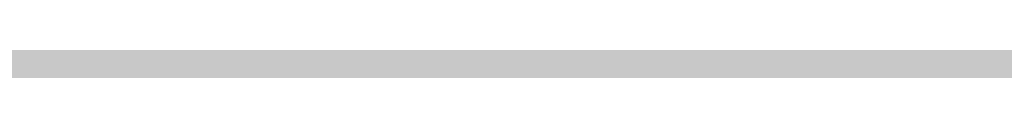
# Model space of a CAD drawing. Units: feet. Extents: x 3168 to 4724, y 827 to 1477.
# Tile 86 of 256: x 3274.148 to 3275.224, y 1099.001 to 1099.015. Entities that reach past the tile are written whole.
import ezdxf

# ---------------------------------------------------------------- set-up
doc = ezdxf.new("R2010")
doc.units = ezdxf.units.FT
doc.layers.add('A-ELEV', color=7, linetype='Continuous', lineweight=35)
doc.layers.add('A-ELEV-PATT', color=8, linetype='Continuous', lineweight=13)

msp = doc.modelspace()

# ---------------------------------------------------------------- hatches: boundary and pattern name
at = {"layer": 'A-ELEV-PATT'}
h = msp.add_hatch(color=256, dxfattribs=at)
h.dxf.hatch_style = 1
edge = h.paths.add_edge_path()
edge.add_ellipse((3552.9058, 979.2201), major_axis=(36.7449, 0), ratio=0.4848485, start_angle=0, end_angle=360)
edge = h.paths.add_edge_path()
edge.add_ellipse((3559.8916, 929.2523), major_axis=(36.7449, 0), ratio=0.4848485, start_angle=0, end_angle=360)
edge = h.paths.add_edge_path()
edge.add_line((3299.3168, 1198.6061), (3479.9167, 1198.6061))
edge.add_line((3479.9167, 1198.6061), (3479.9167, 1209.8686))
edge.add_spline(control_points=[(3479.9167, 1209.8686), (3464.3012, 1209.8686), (3448.6856, 1209.8686), (3410.9491, 1209.8686), (3388.8282, 1209.8686), (3355.6469, 1209.8686), (3344.5864, 1209.8686), (3327.9957, 1209.8686), (3322.4655, 1209.8686), (3314.1702, 1209.8686), (3311.4051, 1209.8686), (3307.2574, 1209.8686), (3305.8748, 1209.8686), (3303.801, 1209.8686), (3303.1097, 1209.8686), (3302.0728, 1209.8686), (3301.7272, 1209.8686), (3301.2087, 1209.8686), (3301.0359, 1209.8686), (3300.7767, 1209.8686), (3300.6903, 1209.8686), (3300.5606, 1209.8686), (3300.5174, 1209.8686), (3300.4526, 1209.8686), (3300.431, 1209.8686), (3300.3986, 1209.8686), (3300.3878, 1209.8686), (3300.3662, 1209.8686), (3300.3457, 1209.8686), (3300.3455, 1209.8686), (3300.3455, 1209.8686), (3300.3433, 1209.8686), (3300.3411, 1209.8686), (3300.3379, 1209.8686), (3300.3368, 1209.8686), (3300.3339, 1209.8686), (3300.3321, 1209.8686), (3300.3255, 1209.8686), (3300.3207, 1209.8686), (3300.3109, 1209.8686), (3300.306, 1209.8686), (3300.2905, 1209.8686), (3300.28, 1209.8686), (3300.2324, 1209.8688), (3300.1953, 1209.869), (3299.9511, 1209.8706), (3299.7448, 1209.8743), (3299.4368, 1209.8833), (3299.3344, 1209.8868), (3299.1811, 1209.8929), (3299.13, 1209.8951), (3298.6522, 1209.9168), (3298.2295, 1209.9457), (3297.6016, 1210.0024), (3297.3934, 1210.0235), (3297.0827, 1210.0583), (3296.9793, 1210.0705), (3296.293, 1210.1549), (3295.7181, 1210.2434), (3294.8687, 1210.3989), (3294.5877, 1210.4545), (3294.1693, 1210.5433), (3294.0304, 1210.5739), (3291.7071, 1211.1012), (3289.6536, 1211.8134), (3285.7763, 1213.564), (3283.9514, 1214.6035), (3280.5122, 1216.9801), (3278.8972, 1218.3176), (3276.3799, 1220.8295), (3275.416, 1221.9177), (3274.0393, 1223.7077), (3273.581, 1224.3495), (3273.1432, 1225.0163)], knot_values=[39.119033, 39.119033, 39.119033, 39.119033, 39.286353, 39.286353, 39.523379, 39.523379, 39.641892, 39.641892, 39.701148, 39.701148, 39.730777, 39.730777, 39.745591, 39.745591, 39.752998, 39.752998, 39.756701, 39.756701, 39.758553, 39.758553, 39.759479, 39.759479, 39.759942, 39.759942, 39.760173, 39.760173, 39.760289, 39.760289, 39.760405, 39.760405, 39.760463, 39.760463, 39.763389, 39.763389, 39.764851, 39.764851, 39.767304, 39.767304, 39.773825, 39.773825, 39.78057, 39.78057, 39.79477, 39.79477, 39.845194, 39.845194, 40.126715, 40.126715, 40.267476, 40.267476, 40.337856, 40.337856, 40.927023, 40.927023, 41.221606, 41.221606, 41.368898, 41.368898, 42.202622, 42.202622, 42.619485, 42.619485, 42.827916, 42.827916, 46.118323, 46.118323, 49.408731, 49.408731, 52.699139, 52.699139, 54.927489, 54.927489, 56.104228, 56.104228, 56.104228, 56.104228], weights=[1, 1, 1, 1, 1, 1, 1, 1, 1, 1, 1, 1, 1, 1, 1, 1, 1, 1, 1, 1, 1, 1, 1, 1, 1, 1, 1, 1, 1, 1, 1, 1, 1, 1, 1, 1, 1, 1, 1, 1, 1, 1, 1, 1, 1, 1, 1, 1, 1, 1, 1, 1, 1, 1, 1, 1, 1, 1, 1, 1, 1, 1, 1, 1, 1, 1, 1, 1, 1, 1, 1, 1, 1, 1], degree=3, periodic=0)
edge.add_line((3273.1432, 1225.0163), (3273.1432, 1099.0163))
edge.add_line((3273.1432, 1099.0163), (3299.3168, 1099.0163))
edge.add_line((3299.3168, 1099.0163), (3299.3168, 1198.6061))
edge = h.paths.add_edge_path()
edge.add_line((3304.7584, 1324.1581), (3479.9167, 1324.1581))
edge.add_line((3479.9167, 1324.1581), (3479.9167, 1335.7146))
edge.add_line((3479.9167, 1335.7146), (3269.1616, 1335.7146))
edge.add_spline(control_points=[(3269.1616, 1335.7146), (3264.0242, 1335.7146), (3258.3641, 1328.9582), (3259.2643, 1323.9003)], knot_values=[0, 0, 0, 0, 15.412191, 15.412191, 15.412191, 15.412191], degree=3, periodic=0)
edge.add_line((3259.2643, 1323.9003), (3265.5168, 1288.7691))
edge.add_line((3265.5168, 1288.7691), (3275.2651, 1261.5456))
edge.add_line((3275.2651, 1261.5456), (3304.7584, 1261.5456))
edge.add_line((3304.7584, 1261.5456), (3304.7584, 1324.1581))
h = msp.add_hatch(color=256, dxfattribs=at)
h.dxf.hatch_style = 1
h.paths.add_polyline_path([(3384.5252, 1099.0163), (3335.0292, 1099.0163), (3299.3168, 1099.0163), (3273.1432, 1099.0163), (3217.5654, 1099.0163), (3168.0693, 827.1163), (3335.0292, 827.1163)])

# ---------------------------------------------------------------- linework, layer by layer
at = {"layer": 'A-ELEV'}
msp.add_open_spline([(3808.5202, 1099.0163), (3808.5202, 1141.4132), (3808.5202, 1183.8102), (3808.5202, 1226.6353), (3808.5202, 1227.0636), (3808.5202, 1227.4918), (3811.4919, 1248.9947), (3814.4635, 1270.4975), (3817.4652, 1292.2176), (3817.4952, 1292.4348), (3817.5253, 1292.652), (3817.5728, 1310.1067), (3817.6203, 1327.5615), (3817.6679, 1345.0163), (3817.6679, 1345.458), (3817.6679, 1345.8996), (3817.6679, 1346.456), (3817.6679, 1346.5708), (3817.6679, 1346.7529), (3817.6679, 1346.8201), (3817.6679, 1346.9349), (3817.6679, 1346.9823), (3817.6679, 1347.0386), (3817.6679, 1347.0474), (3817.6679, 1347.0737), (3817.6679, 1347.0593), (3817.6679, 1347.0615), (3817.6679, 1347.0627), (3817.6679, 1347.066), (3817.6679, 1347.0683), (3817.6679, 1347.075), (3817.6679, 1347.0795), (3817.6678, 1347.0929), (3817.6678, 1347.1019), (3817.6678, 1347.1288), (3817.6677, 1347.1467), (3817.6674, 1347.2004), (3817.6672, 1347.2362), (3817.6661, 1347.3434), (3817.665, 1347.4147), (3817.6608, 1347.6281), (3817.6566, 1347.7697), (3817.64, 1348.1925), (3817.6235, 1348.4716), (3817.5591, 1349.3001), (3817.4961, 1349.8406), (3817.2554, 1351.4242), (3817.0263, 1352.4288), (3816.3069, 1354.8889), (3815.7437, 1356.2687), (3814.464, 1358.8192), (3813.7464, 1359.991), (3812.1958, 1362.1723), (3811.3622, 1363.1821), (3809.5888, 1365.069), (3808.6488, 1365.9461), (3806.6543, 1367.5796), (3805.5997, 1368.3362), (3803.3529, 1369.7223), (3802.1605, 1370.3524), (3799.6008, 1371.4536), (3798.2327, 1371.9255), (3795.2801, 1372.6346), (3793.6931, 1372.8721), (3791.8694, 1372.9265), (3791.7409, 1372.9292), (3791.3534, 1372.9341), (3791.0927, 1372.9329), (3790.3041, 1372.9151), (3789.7695, 1372.8842), (3789.2092, 1372.8302), (3789.1906, 1372.8284), (3789.1349, 1372.8229), (3789.0977, 1372.8191), (3789.0484, 1372.814), (3789.0364, 1372.8127), (3789.0003, 1372.8089), (3788.9761, 1372.8063), (3788.9494, 1372.8034), (3788.9468, 1372.8031), (3788.9426, 1372.8027), (3788.941, 1372.8025), (3788.9386, 1372.8022), (3788.9378, 1372.8021), (3788.9354, 1372.8019), (3788.8675, 1372.7944), (3788.7569, 1372.7822), (3788.7015, 1372.7761), (3788.5355, 1372.7579), (3788.4249, 1372.7457), (3788.0929, 1372.7092), (3787.8715, 1372.6848), (3787.2075, 1372.6118), (3786.7648, 1372.5631), (3785.4368, 1372.417), (3784.5515, 1372.3196), (3781.8954, 1372.0274), (3780.1247, 1371.8327), (3774.8126, 1371.2483), (3771.2713, 1370.8587), (3760.6471, 1369.69), (3753.5643, 1368.9109), (3732.316, 1366.5735), (3718.1504, 1365.0152), (3694.0068, 1362.3593), (3684.0287, 1361.2617), (3674.0506, 1360.1641), (3664.6007, 1360.1641), (3655.1508, 1360.1641), (3626.8011, 1360.1641), (3607.9013, 1360.1641), (3551.2019, 1360.1641), (3513.4023, 1360.1641), (3467.7252, 1360.1641), (3459.8476, 1360.1641), (3436.2149, 1360.1641), (3420.4597, 1360.1641), (3373.1943, 1360.1641), (3341.6839, 1360.1641), (3302.8482, 1360.1641), (3295.5227, 1360.1641), (3286.0383, 1360.1641), (3283.8794, 1360.1641), (3277.4026, 1360.1641), (3273.0848, 1360.1641), (3267.7329, 1360.1641), (3266.6988, 1360.1641), (3263.5965, 1360.1641), (3261.5284, 1360.1641), (3259.2369, 1360.1641), (3259.0137, 1360.1641), (3258.344, 1360.1641), (3257.8975, 1360.1641), (3257.431, 1360.1641), (3257.411, 1360.1641), (3257.3706, 1360.1641), (3257.3755, 1360.1641), (3257.3746, 1360.1641), (3257.3739, 1360.1641), (3257.372, 1360.1641), (3257.3706, 1360.1641), (3257.3667, 1360.1641), (3257.364, 1360.1641), (3257.3561, 1360.1641), (3257.3508, 1360.164), (3257.335, 1360.164), (3257.3244, 1360.164), (3257.2928, 1360.1639), (3257.2717, 1360.1638), (3257.2084, 1360.1634), (3257.1663, 1360.163), (3257.0402, 1360.1614), (3256.9563, 1360.1598), (3256.7055, 1360.1534), (3256.5392, 1360.147), (3256.0436, 1360.1219), (3255.7173, 1360.0971), (3254.7524, 1360.0005), (3254.128, 1359.9065), (3252.1801, 1359.5253), (3250.9416, 1359.144), (3248.6702, 1358.2433), (3247.6357, 1357.7238), (3245.7326, 1356.6035), (3244.8634, 1356.0021), (3243.2531, 1354.7429), (3242.512, 1354.0847), (3240.7511, 1352.3448), (3239.801, 1351.2296), (3238.0878, 1348.8724), (3237.3247, 1347.6304), (3235.9825, 1344.9716), (3235.4022, 1343.5549), (3234.5911, 1340.8155), (3234.3109, 1339.5435), (3233.9765, 1336.8026), (3233.9221, 1335.3309), (3234.1489, 1332.5913), (3234.3495, 1331.3672), (3234.7199, 1329.9994), (3234.7524, 1329.8834), (3234.8536, 1329.5348), (3234.9259, 1329.3017), (3235.0248, 1329.0026), (3235.0469, 1328.9369), (3235.0776, 1328.8472), (3235.0859, 1328.8232), (3235.1109, 1328.7511), (3235.1278, 1328.703), (3235.148, 1328.6462), (3235.1511, 1328.6376), (3235.1561, 1328.6235), (3235.1581, 1328.618), (3235.1602, 1328.612), (3235.1656, 1328.5969), (3235.1801, 1328.5565), (3235.1903, 1328.5281), (3235.2208, 1328.4429), (3235.2411, 1328.3862), (3235.3021, 1328.2159), (3235.3427, 1328.1023), (3235.4647, 1327.7617), (3235.546, 1327.5346), (3235.79, 1326.8534), (3235.9526, 1326.3992), (3236.4405, 1325.0367), (3236.7657, 1324.1284), (3237.7415, 1321.4034), (3238.392, 1319.5868), (3240.3435, 1314.1369), (3241.6445, 1310.5036), (3245.5476, 1299.6037), (3248.1496, 1292.3371), (3255.9557, 1270.5374), (3261.1598, 1256.0042), (3267.3876, 1238.612), (3268.4114, 1235.7529), (3269.5104, 1232.6839), (3269.5856, 1232.4739), (3269.7066, 1232.1359), (3269.7524, 1232.0079), (3269.8273, 1231.7987), (3269.8564, 1231.7176), (3269.9063, 1231.5781), (3269.9272, 1231.5198), (3269.9725, 1231.3934), (3269.9968, 1231.3254), (3270.0265, 1231.2425), (3270.0318, 1231.2277), (3270.0403, 1231.204), (3270.0392, 1231.207), (3270.0394, 1231.2066), (3270.0394, 1231.2064), (3270.0396, 1231.2058), (3270.0398, 1231.2055), (3270.0402, 1231.2043), (3270.0404, 1231.2036), (3270.0413, 1231.2013), (3270.0418, 1231.1998), (3270.0434, 1231.1953), (3270.0445, 1231.1922), (3270.0478, 1231.1832), (3270.0499, 1231.1771), (3270.0564, 1231.159), (3270.0608, 1231.147), (3270.0739, 1231.1108), (3270.0826, 1231.0867), (3270.1089, 1231.0144), (3270.1266, 1230.9663), (3270.1799, 1230.8225), (3270.2159, 1230.7269), (3270.3253, 1230.4415), (3270.4, 1230.2528), (3270.6292, 1229.6914), (3270.7889, 1229.3235), (3271.2865, 1228.2383), (3271.6431, 1227.5398), (3272.7759, 1225.5153), (3273.6142, 1224.2605), (3275.416, 1221.9177), (3276.3799, 1220.8295), (3278.8972, 1218.3176), (3280.5122, 1216.9801), (3283.9514, 1214.6035), (3285.7763, 1213.564), (3289.6536, 1211.8134), (3291.7071, 1211.1012), (3294.0304, 1210.5739), (3294.1693, 1210.5433), (3294.5877, 1210.4545), (3294.8687, 1210.3989), (3295.7181, 1210.2434), (3296.293, 1210.1549), (3296.9793, 1210.0705), (3297.0827, 1210.0583), (3297.3934, 1210.0235), (3297.6016, 1210.0024), (3298.2295, 1209.9457), (3298.6522, 1209.9168), (3299.13, 1209.8951), (3299.1811, 1209.8929), (3299.3344, 1209.8868), (3299.4368, 1209.8833), (3299.7448, 1209.8743), (3299.9511, 1209.8706), (3300.1953, 1209.869), (3300.2324, 1209.8688), (3300.28, 1209.8686), (3300.2905, 1209.8686), (3300.306, 1209.8686), (3300.3109, 1209.8686), (3300.3207, 1209.8686), (3300.3255, 1209.8686), (3300.3321, 1209.8686), (3300.3339, 1209.8686), (3300.3368, 1209.8686), (3300.3379, 1209.8686), (3300.3411, 1209.8686), (3300.3433, 1209.8686), (3300.3455, 1209.8686), (3300.3455, 1209.8686), (3300.3457, 1209.8686), (3300.3662, 1209.8686), (3300.3878, 1209.8686), (3300.3986, 1209.8686), (3300.431, 1209.8686), (3300.4526, 1209.8686), (3300.5174, 1209.8686), (3300.5606, 1209.8686), (3300.6903, 1209.8686), (3300.7767, 1209.8686), (3301.0359, 1209.8686), (3301.2087, 1209.8686), (3301.7272, 1209.8686), (3302.0728, 1209.8686), (3303.1097, 1209.8686), (3303.801, 1209.8686), (3305.8748, 1209.8686), (3307.2574, 1209.8686), (3311.4051, 1209.8686), (3314.1702, 1209.8686), (3322.4655, 1209.8686), (3327.9957, 1209.8686), (3344.5864, 1209.8686), (3355.6469, 1209.8686), (3388.8282, 1209.8686), (3410.9491, 1209.8686), (3477.3119, 1209.8686), (3521.5537, 1209.8686), (3566.8362, 1209.8686), (3567.8769, 1209.8686), (3570.999, 1209.8686), (3573.0804, 1209.8686), (3575.7814, 1209.8686), (3576.4009, 1209.8686), (3577.2958, 1209.8686), (3577.5712, 1209.8686), (3578.3971, 1209.8686), (3578.9478, 1209.8686), (3579.7565, 1209.8686), (3580.0145, 1209.8686), (3580.3427, 1209.8686), (3580.3269, 1209.8686), (3580.3272, 1209.8686), (3580.3273, 1209.8686), (3580.3278, 1209.8686), (3580.3281, 1209.8686), (3580.329, 1209.8686), (3580.3296, 1209.8686), (3580.3314, 1209.8686), (3580.3327, 1209.8686), (3580.3363, 1209.8686), (3580.3388, 1209.8686), (3580.3461, 1209.8686), (3580.351, 1209.8686), (3580.3657, 1209.8685), (3580.3754, 1209.8685), (3580.4048, 1209.8684), (3580.4244, 1209.8684), (3580.4832, 1209.8681), (3580.5224, 1209.8678), (3580.6404, 1209.8666), (3580.7192, 1209.8655), (3580.9563, 1209.8608), (3581.1152, 1209.8561), (3581.5942, 1209.8372), (3581.9164, 1209.8183), (3582.8899, 1209.7424), (3583.548, 1209.6662), (3585.5318, 1209.3606), (3586.8672, 1209.0539), (3589.4715, 1208.2525), (3590.7402, 1207.7579), (3591.9955, 1207.1588), (3592.0578, 1207.1287), (3592.2442, 1207.038), (3592.3677, 1206.9766), (3592.7353, 1206.7904), (3592.9768, 1206.6631), (3593.2445, 1206.5164), (3593.2747, 1206.4998), (3593.3651, 1206.4498), (3593.4251, 1206.4163), (3593.6043, 1206.3153), (3593.7227, 1206.2472), (3593.8572, 1206.1684), (3593.8744, 1206.1583), (3593.9257, 1206.128), (3593.9599, 1206.1078), (3594.0621, 1206.0469), (3594.1298, 1206.0061), (3594.2084, 1205.9582), (3594.2197, 1205.9513), (3594.2534, 1205.9307), (3594.2758, 1205.9169), (3594.343, 1205.8755), (3594.3876, 1205.8479), (3594.4336, 1205.819), (3594.4353, 1205.818), (3594.4402, 1205.8149), (3594.4435, 1205.8129), (3594.4471, 1205.8106), (3594.4475, 1205.8103), (3594.4487, 1205.8096), (3594.4495, 1205.8091), (3594.4504, 1205.8086), (3594.4505, 1205.8085), (3594.4506, 1205.8084), (3594.4674, 1205.7979), (3594.4933, 1205.7817), (3594.5062, 1205.7736), (3594.545, 1205.7492), (3594.5709, 1205.733), (3594.6485, 1205.6844), (3594.7002, 1205.652), (3594.8554, 1205.5547), (3594.9589, 1205.4898), (3595.2694, 1205.2953), (3595.4763, 1205.1656), (3596.0972, 1204.7765), (3596.5111, 1204.5171), (3597.7528, 1203.7388), (3598.5807, 1203.22), (3601.0642, 1201.6636), (3602.7198, 1200.6259), (3607.6868, 1197.513), (3610.9981, 1195.4377), (3620.932, 1189.2119), (3627.5546, 1185.0614), (3647.4225, 1172.6097), (3660.6678, 1164.3086), (3700.4035, 1139.4053), (3726.894, 1122.8031), (3757.2057, 1103.8061), (3761.027, 1101.4112), (3764.8482, 1099.0163), (3745.3283, 1099.0163), (3725.8083, 1099.0163), (3706.2884, 1099.0163), (3706.2884, 1108.4532), (3706.2884, 1117.8902), (3706.2884, 1127.3271), (3710.7508, 1127.3271), (3715.2131, 1127.3271), (3719.6755, 1127.3271)], degree=3, knots=[0, 0, 0, 0, 0.982037, 0.982037, 0.991957, 0.991957, 0.991957, 1.966522, 1.966522, 1.976367, 1.976367, 1.976367, 2.976367, 2.976367, 2.976367, 3.00169, 3.00169, 3.008272, 3.008272, 3.012129, 3.012129, 3.014851, 3.014851, 3.015353, 3.015353, 3.016359, 3.016359, 3.017365, 3.017365, 3.019376, 3.019376, 3.023398, 3.023398, 3.031442, 3.031442, 3.047531, 3.047531, 3.079708, 3.079708, 3.144063, 3.144063, 3.272772, 3.272772, 3.53019, 3.53019, 4.045026, 4.045026, 5.074698, 5.074698, 6.700878, 6.700878, 8.327058, 8.327058, 9.953238, 9.953238, 11.579418, 11.579418, 13.205598, 13.205598, 14.831778, 14.831778, 16.457958, 16.457958, 18.084138, 18.084138, 18.206872, 18.206872, 18.45234, 18.45234, 18.943275, 18.943275, 18.960093, 18.960093, 18.993729, 18.993729, 19.00461, 19.00461, 19.026374, 19.026374, 19.028737, 19.028737, 19.03018, 19.03018, 19.030897, 19.030897, 19.032332, 19.032332, 19.033766, 19.033766, 19.036636, 19.036636, 19.042374, 19.042374, 19.053851, 19.053851, 19.076805, 19.076805, 19.122714, 19.122714, 19.21453, 19.21453, 19.398163, 19.398163, 19.765429, 19.765429, 20.024128, 20.024128, 20.024128, 20.092031, 20.092031, 20.227836, 20.227836, 20.499446, 20.499446, 20.556051, 20.556051, 20.66926, 20.66926, 20.895678, 20.895678, 20.948316, 20.948316, 20.963829, 20.963829, 20.994855, 20.994855, 21.002285, 21.002285, 21.017146, 21.017146, 21.01875, 21.01875, 21.021959, 21.021959, 21.022102, 21.022102, 21.022249, 21.022249, 21.022708, 21.022708, 21.023627, 21.023627, 21.025464, 21.025464, 21.029138, 21.029138, 21.036486, 21.036486, 21.051183, 21.051183, 21.080575, 21.080575, 21.139361, 21.139361, 21.256932, 21.256932, 21.492073, 21.492073, 21.962356, 21.962356, 23.01002, 23.01002, 24.057684, 24.057684, 25.105348, 25.105348, 26.153011, 26.153011, 27.776787, 27.776787, 29.400562, 29.400562, 31.024337, 31.024337, 32.278801, 32.278801, 33.533265, 33.533265, 34.467568, 34.467568, 34.553971, 34.553971, 34.726776, 34.726776, 34.775309, 34.775309, 34.793079, 34.793079, 34.82862, 34.82862, 34.834979, 34.834979, 34.839039, 34.839039, 34.839411, 34.839411, 34.840285, 34.840285, 34.842034, 34.842034, 34.845531, 34.845531, 34.852525, 34.852525, 34.866512, 34.866512, 34.894488, 34.894488, 34.950439, 34.950439, 35.062342, 35.062342, 35.286147, 35.286147, 35.733758, 35.733758, 35.821815, 35.821815, 35.828283, 35.828283, 35.832225, 35.832225, 35.834724, 35.834724, 35.836521, 35.836521, 35.838617, 35.838617, 35.839073, 35.839073, 35.839345, 35.839345, 35.839617, 35.839617, 35.840161, 35.840161, 35.841249, 35.841249, 35.843425, 35.843425, 35.847778, 35.847778, 35.856482, 35.856482, 35.873891, 35.873891, 35.908709, 35.908709, 35.978345, 35.978345, 36.117617, 36.117617, 36.396161, 36.396161, 36.953248, 36.953248, 38.067423, 38.067423, 40.295772, 40.295772, 42.524122, 42.524122, 45.81453, 45.81453, 49.104937, 49.104937, 52.395345, 52.395345, 52.603776, 52.603776, 53.020639, 53.020639, 53.854363, 53.854363, 54.001655, 54.001655, 54.296238, 54.296238, 54.885405, 54.885405, 54.955785, 54.955785, 55.096546, 55.096546, 55.378067, 55.378067, 55.42849, 55.42849, 55.442691, 55.442691, 55.449436, 55.449436, 55.455957, 55.455957, 55.458409, 55.458409, 55.459872, 55.459872, 55.462798, 55.462798, 55.462856, 55.462856, 55.462972, 55.462972, 55.463088, 55.463088, 55.463319, 55.463319, 55.463782, 55.463782, 55.464708, 55.464708, 55.46656, 55.46656, 55.470263, 55.470263, 55.47767, 55.47767, 55.492484, 55.492484, 55.522112, 55.522112, 55.581369, 55.581369, 55.699882, 55.699882, 55.936907, 55.936907, 56.410959, 56.410959, 56.42211, 56.42211, 56.444413, 56.444413, 56.451051, 56.451051, 56.454001, 56.454001, 56.459901, 56.459901, 56.462666, 56.462666, 56.463418, 56.463418, 56.464171, 56.464171, 56.465675, 56.465675, 56.468684, 56.468684, 56.474702, 56.474702, 56.486738, 56.486738, 56.51081, 56.51081, 56.558955, 56.558955, 56.655243, 56.655243, 56.847821, 56.847821, 57.232975, 57.232975, 58.003284, 58.003284, 59.543901, 59.543901, 62.625137, 62.625137, 68.787607, 68.787607, 74.950078, 74.950078, 75.27336, 75.27336, 75.919923, 75.919923, 77.213051, 77.213051, 77.377769, 77.377769, 77.707206, 77.707206, 78.366079, 78.366079, 78.462532, 78.462532, 78.655436, 78.655436, 79.041245, 79.041245, 79.105735, 79.105735, 79.234714, 79.234714, 79.492672, 79.492672, 79.502197, 79.502197, 79.521249, 79.521249, 79.523534, 79.523534, 79.528103, 79.528103, 79.528682, 79.528682, 79.528885, 79.528885, 79.529089, 79.529089, 79.529495, 79.529495, 79.530308, 79.530308, 79.531935, 79.531935, 79.535187, 79.535187, 79.541693, 79.541693, 79.554704, 79.554704, 79.580725, 79.580725, 79.632769, 79.632769, 79.736856, 79.736856, 79.94503, 79.94503, 80.361377, 80.361377, 80.421435, 80.421435, 80.421435, 81.421435, 81.421435, 81.421435, 82.421435, 82.421435, 82.421435, 83.421435, 83.421435, 83.421435, 83.421435], dxfattribs=at)

doc.saveas('drawing.dxf')
